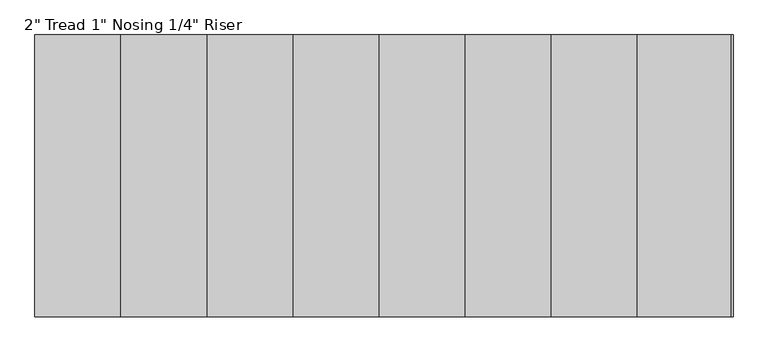
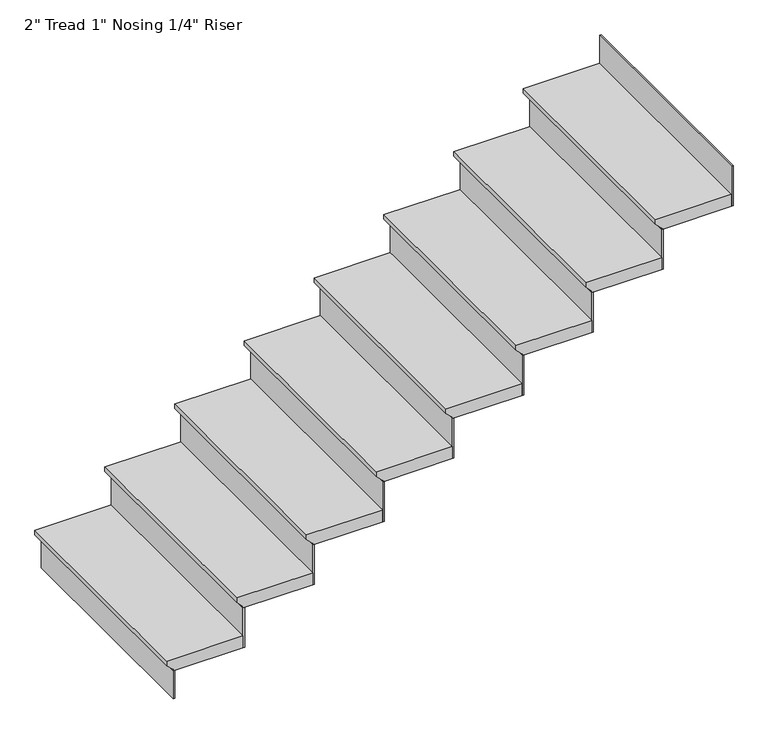
"""IFC4 building model written with IfcOpenShell, lengths in millimetres: stair flight geometry."""

from ifc_helpers import new_model, si_unit, frame, origin, origin_with_axes, place, context, project, spatial, polyline, outline, extrude, source, transform, mapped, element, save


def stair_flight_77e6af34(model_context):
    return source(origin(), model_context, "Body", "SweptSolid", [
        extrude(outline(polyline([(169.3333333, -5642.9873398), (169.3333333, -5947.7873398), (150.2833333, -5947.7873398), (124.8833333, -5922.3873398), (118.5333333, -5922.3873398), (118.5333333, -5642.9873398), (169.3333333, -5642.9873398)])), frame((0.0, 908.7549175, 0.0), z_axis=(0.0, 1.0, 0.0), x_axis=(0.0, 0.0, 1.0)), (0.0, 0.0, 1.0), 914.4),
        extrude(outline(polyline([(-5916.0373398, 908.7549175), (-5922.3873398, 908.7549175), (-5922.3873398, 1823.1549175), (-5916.0373398, 1823.1549175), (-5916.0373398, 908.7549175)])), origin_with_axes(), (0.0, 0.0, 1.0), 118.5333333),
        extrude(outline(polyline([(-5636.6373398, 908.7549175), (-5642.9873398, 908.7549175), (-5642.9873398, 1823.1549175), (-5636.6373398, 1823.1549175), (-5636.6373398, 908.7549175)])), frame((0.0, 0.0, 118.5333333), z_axis=(0.0, 0.0, 1.0), x_axis=(1.0, 0.0, 0.0)), (0.0, 0.0, 1.0), 169.3333333),
        extrude(outline(polyline([(338.6666667, -5363.5873398), (338.6666667, -5668.3873398), (319.6166667, -5668.3873398), (294.2166667, -5642.9873398), (287.8666667, -5642.9873398), (287.8666667, -5363.5873398), (338.6666667, -5363.5873398)])), frame((0.0, 908.7549175, 0.0), z_axis=(0.0, 1.0, 0.0), x_axis=(0.0, 0.0, 1.0)), (0.0, 0.0, 1.0), 914.4),
        extrude(outline(polyline([(-5357.2373398, 908.7549175), (-5363.5873398, 908.7549175), (-5363.5873398, 1823.1549175), (-5357.2373398, 1823.1549175), (-5357.2373398, 908.7549175)])), frame((0.0, 0.0, 287.8666667), z_axis=(0.0, 0.0, 1.0), x_axis=(1.0, 0.0, 0.0)), (0.0, 0.0, 1.0), 169.3333333),
        extrude(outline(polyline([(508.0, -5084.1873398), (508.0, -5388.9873398), (488.95, -5388.9873398), (463.55, -5363.5873398), (457.2, -5363.5873398), (457.2, -5084.1873398), (508.0, -5084.1873398)])), frame((0.0, 908.7549175, 0.0), z_axis=(0.0, 1.0, 0.0), x_axis=(0.0, 0.0, 1.0)), (0.0, 0.0, 1.0), 914.4),
        extrude(outline(polyline([(-5077.8373398, 908.7549175), (-5084.1873398, 908.7549175), (-5084.1873398, 1823.1549175), (-5077.8373398, 1823.1549175), (-5077.8373398, 908.7549175)])), frame((0.0, 0.0, 457.2), z_axis=(0.0, 0.0, 1.0), x_axis=(1.0, 0.0, 0.0)), (0.0, 0.0, 1.0), 169.3333333),
        extrude(outline(polyline([(677.3333333, -4804.7873398), (677.3333333, -5109.5873398), (658.2833333, -5109.5873398), (632.8833333, -5084.1873398), (626.5333333, -5084.1873398), (626.5333333, -4804.7873398), (677.3333333, -4804.7873398)])), frame((0.0, 908.7549175, 0.0), z_axis=(0.0, 1.0, 0.0), x_axis=(0.0, 0.0, 1.0)), (0.0, 0.0, 1.0), 914.4),
        extrude(outline(polyline([(-4798.4373398, 908.7549175), (-4804.7873398, 908.7549175), (-4804.7873398, 1823.1549175), (-4798.4373398, 1823.1549175), (-4798.4373398, 908.7549175)])), frame((0.0, 0.0, 626.5333333), z_axis=(0.0, 0.0, 1.0), x_axis=(1.0, 0.0, 0.0)), (0.0, 0.0, 1.0), 169.3333333),
        extrude(outline(polyline([(846.6666667, -4525.3873398), (846.6666667, -4830.1873398), (827.6166667, -4830.1873398), (802.2166667, -4804.7873398), (795.8666667, -4804.7873398), (795.8666667, -4525.3873398), (846.6666667, -4525.3873398)])), frame((0.0, 908.7549175, 0.0), z_axis=(0.0, 1.0, 0.0), x_axis=(0.0, 0.0, 1.0)), (0.0, 0.0, 1.0), 914.4),
        extrude(outline(polyline([(-4519.0373398, 908.7549175), (-4525.3873398, 908.7549175), (-4525.3873398, 1823.1549175), (-4519.0373398, 1823.1549175), (-4519.0373398, 908.7549175)])), frame((0.0, 0.0, 795.8666667), z_axis=(0.0, 0.0, 1.0), x_axis=(1.0, 0.0, 0.0)), (0.0, 0.0, 1.0), 169.3333333),
        extrude(outline(polyline([(1016.0, -4245.9873398), (1016.0, -4550.7873398), (996.95, -4550.7873398), (971.55, -4525.3873398), (965.2, -4525.3873398), (965.2, -4245.9873398), (1016.0, -4245.9873398)])), frame((0.0, 908.7549175, 0.0), z_axis=(0.0, 1.0, 0.0), x_axis=(0.0, 0.0, 1.0)), (0.0, 0.0, 1.0), 914.4),
        extrude(outline(polyline([(-4239.6373398, 908.7549175), (-4245.9873398, 908.7549175), (-4245.9873398, 1823.1549175), (-4239.6373398, 1823.1549175), (-4239.6373398, 908.7549175)])), frame((0.0, 0.0, 965.2), z_axis=(0.0, 0.0, 1.0), x_axis=(1.0, 0.0, 0.0)), (0.0, 0.0, 1.0), 169.3333333),
        extrude(outline(polyline([(1185.3333333, -3966.5873398), (1185.3333333, -4271.3873398), (1166.2833333, -4271.3873398), (1140.8833333, -4245.9873398), (1134.5333333, -4245.9873398), (1134.5333333, -3966.5873398), (1185.3333333, -3966.5873398)])), frame((0.0, 908.7549175, 0.0), z_axis=(0.0, 1.0, 0.0), x_axis=(0.0, 0.0, 1.0)), (0.0, 0.0, 1.0), 914.4),
        extrude(outline(polyline([(-3960.2373398, 908.7549175), (-3966.5873398, 908.7549175), (-3966.5873398, 1823.1549175), (-3960.2373398, 1823.1549175), (-3960.2373398, 908.7549175)])), frame((0.0, 0.0, 1134.5333333), z_axis=(0.0, 0.0, 1.0), x_axis=(1.0, 0.0, 0.0)), (0.0, 0.0, 1.0), 169.3333333),
        extrude(outline(polyline([(-3680.8373398, 908.7549175), (-3687.1873398, 908.7549175), (-3687.1873398, 1823.1549175), (-3680.8373398, 1823.1549175), (-3680.8373398, 908.7549175)])), frame((0.0, 0.0, 1303.8666667), z_axis=(0.0, 0.0, 1.0), x_axis=(1.0, 0.0, 0.0)), (0.0, 0.0, 1.0), 169.3333333),
        extrude(outline(polyline([(1354.6666667, -3687.1873398), (1354.6666667, -3991.9873398), (1335.6166667, -3991.9873398), (1310.2166667, -3966.5873398), (1303.8666667, -3966.5873398), (1303.8666667, -3687.1873398), (1354.6666667, -3687.1873398)])), frame((0.0, 908.7549175, 0.0), z_axis=(0.0, 1.0, 0.0), x_axis=(0.0, 0.0, 1.0)), (0.0, 0.0, 1.0), 914.4),
    ])


if __name__ == "__main__":
    model = new_model("IFC4")
    model_context = context("Model", 3, world=origin())
    ifc_project = project(units=[si_unit("LENGTHUNIT", "METRE", prefix="MILLI")], contexts=[model_context])
    site = spatial("IfcSite", under=ifc_project)
    building = spatial("IfcBuilding", under=site)
    placement = place(None, origin())
    stair_flight_shape = stair_flight_77e6af34(model_context)
    element("IfcStairFlight", 1, ObjectType="2\" Tread 1\" Nosing 1/4\" Riser", at=placement, inside=building, context=model_context, shape_type="MappedRepresentation", body=[
        mapped(stair_flight_shape, transform((0.0, 0.0, 0.0), x_axis=(1.0, 0.0, 0.0), y_axis=(0.0, 1.0, 0.0), z_axis=(0.0, 0.0, 1.0))),
    ])
    save(model, "model.ifc")
